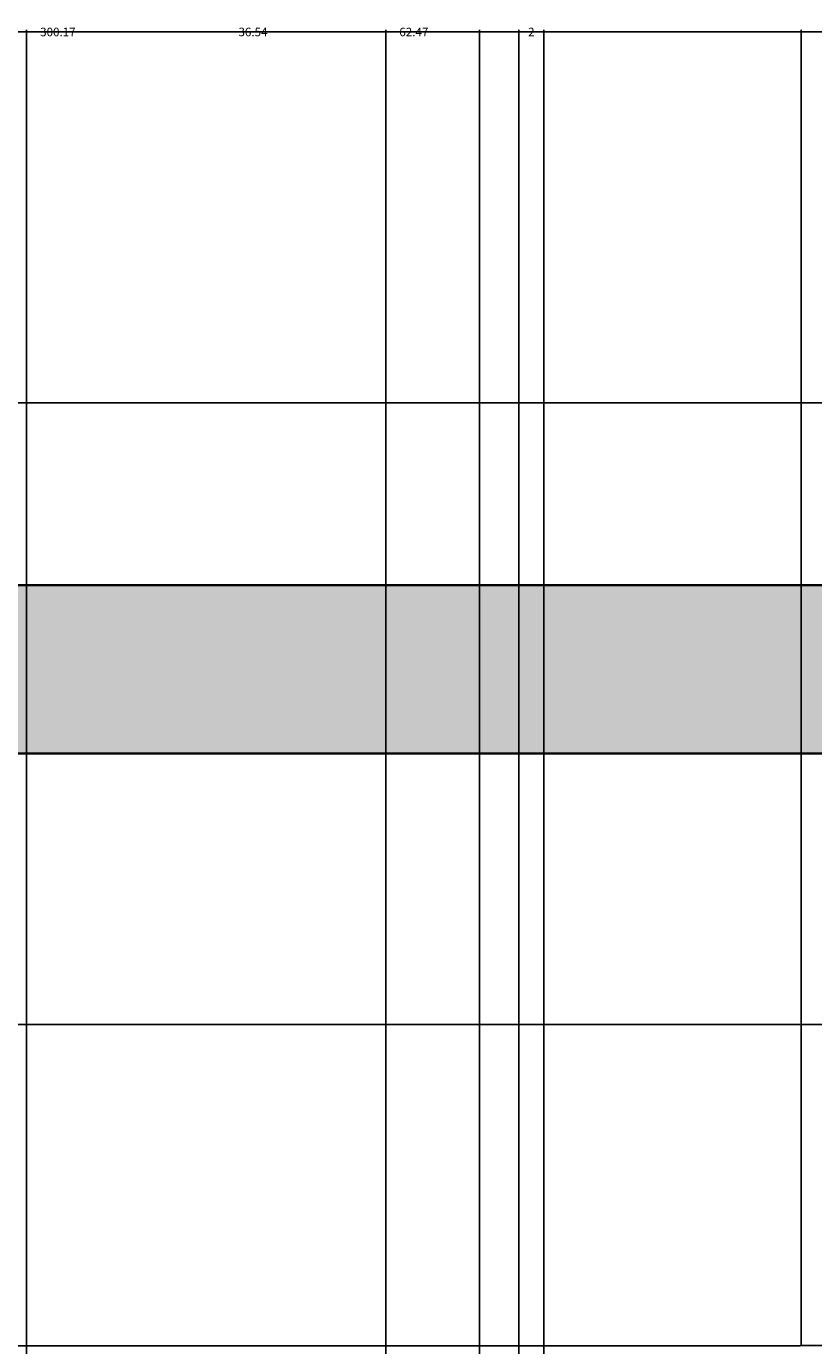
# Model space of a CAD drawing. Units: inches. Extents: x -145 to 510, y 5 to 386.
# Tile 21 of 25: x 182 to 245, y 280 to 386. Entities that reach past the tile are written whole.
import ezdxf

# ---------------------------------------------------------------- set-up
doc = ezdxf.new("R2010")
doc.units = ezdxf.units.IN
doc.header["$MEASUREMENT"] = 0
for name, color, linetype, lineweight in [('A-ANNO-DIMS', 2, 'Continuous', 18), ('A-ELEV', 7, 'Continuous', 35), ('A-ELEV-PATT', 8, 'Continuous', 13), ('A-GLAZ', 4, 'Continuous', 25)]:
    doc.layers.add(name, color=color, linetype=linetype, lineweight=lineweight)
doc.styles.get("Standard").update_dxf_attribs({"font": 'arial.ttf'})
doc.dimstyles.get("Standard").update_dxf_attribs({"dimtxt": 0.6875, "dimasz": 0.18, "dimexe": 0.18, "dimexo": 0.0625, "dimgap": 0.09, "dimtad": 0, "dimtih": 1, "dimtoh": 1, "dimdec": 4, "dimzin": 0, "dimdsep": 46, "dimlunit": 4, "dimtxsty": 'Standard', "dimcen": 0.09, "dimadec": 0, "dimazin": 0, "dimtfac": 1, "dimtdec": 4, "dimtofl": 0, "dimtmove": 0, "dimatfit": 3, "dimfxl": 1, "dimtolj": 1, "dimtzin": 0, "dimarcsym": 0})

# ---------------------------------------------------------------- blocks, each defined once
blk = doc.blocks.new('*D14')
at = {"layer": 'A-ANNO-DIMS', "color": 0, "lineweight": -2, "transparency": 16777216}
for p, q in [((34.27, 341.23), (34.27, 385.97)), ((34.45, 385.79), (255.28, 385.79)), ((478.65, 385.79), (257.81, 385.79)), ((478.83, 355.95), (478.83, 385.97))]:
    blk.add_line(p, q, dxfattribs=at)
at = {"layer": 'A-ANNO-DIMS', "color": 0, "transparency": 16777216}
for points in [[(34.45, 385.82), (34.45, 385.76), (34.27, 385.79)], [(478.65, 385.82), (478.65, 385.76), (478.83, 385.79)]]:
    blk.add_solid(points, dxfattribs=at)
at = {"layer": 'Defpoints', "color": 0, "transparency": 16777216}
for p in [(478.83, 385.79), (478.83, 355.89), (34.27, 341.17)]:
    blk.add_point(p, dxfattribs=at)
at = {"layer": 'A-ANNO-DIMS', "color": 0, "transparency": 16777216, "insert": (256.55, 385.79), "char_height": 0.688, "attachment_point": 5}
blk.add_mtext('\\A1;444.6', dxfattribs=at)
blk = doc.blocks.new('*D16')
at = {"layer": 'A-ANNO-DIMS', "color": 0, "lineweight": -2, "transparency": 16777216}
for p, q in [((95.14, 305.8), (95.14, 385.97)), ((95.32, 385.79), (137.23, 385.79)), ((181.64, 385.79), (139.73, 385.79)), ((181.82, 305.8), (181.82, 385.97))]:
    blk.add_line(p, q, dxfattribs=at)
at = {"layer": 'A-ANNO-DIMS', "color": 0, "transparency": 16777216}
for points in [[(95.32, 385.82), (95.32, 385.76), (95.14, 385.79)], [(181.64, 385.82), (181.64, 385.76), (181.82, 385.79)]]:
    blk.add_solid(points, dxfattribs=at)
at = {"layer": 'Defpoints', "color": 0, "transparency": 16777216}
for p in [(181.82, 385.79), (95.14, 305.74), (181.82, 305.74)]:
    blk.add_point(p, dxfattribs=at)
at = {"layer": 'A-ANNO-DIMS', "color": 0, "transparency": 16777216, "insert": (138.48, 385.79), "char_height": 0.688, "attachment_point": 5}
blk.add_mtext('\\A1;86.68', dxfattribs=at)
blk = doc.blocks.new('*D17')
at = {"layer": 'A-ANNO-DIMS', "color": 0, "lineweight": -2, "transparency": 16777216}
for p, q in [((181.82, 305.8), (181.82, 385.97)), ((182, 385.79), (211.8, 385.79)), ((244.11, 385.79), (214.31, 385.79)), ((244.29, 305.8), (244.29, 385.97))]:
    blk.add_line(p, q, dxfattribs=at)
at = {"layer": 'A-ANNO-DIMS', "color": 0, "transparency": 16777216}
for points in [[(182, 385.82), (182, 385.76), (181.82, 385.79)], [(244.11, 385.82), (244.11, 385.76), (244.29, 385.79)]]:
    blk.add_solid(points, dxfattribs=at)
at = {"layer": 'Defpoints', "color": 0, "transparency": 16777216}
for p in [(244.29, 385.79), (181.82, 305.74), (244.29, 305.74)]:
    blk.add_point(p, dxfattribs=at)
at = {"layer": 'A-ANNO-DIMS', "color": 0, "transparency": 16777216, "insert": (213.06, 385.79), "char_height": 0.688, "attachment_point": 5}
blk.add_mtext('\\A1;62.47', dxfattribs=at)
blk = doc.blocks.new('*D18')
at = {"layer": 'A-ANNO-DIMS', "color": 0, "lineweight": -2, "transparency": 16777216}
for p, q in [((244.29, 305.8), (244.29, 385.97)), ((244.47, 385.79), (268.26, 385.79)), ((294.56, 385.79), (270.77, 385.79)), ((294.74, 305.8), (294.74, 385.97))]:
    blk.add_line(p, q, dxfattribs=at)
at = {"layer": 'A-ANNO-DIMS', "color": 0, "transparency": 16777216}
for points in [[(244.47, 385.82), (244.47, 385.76), (244.29, 385.79)], [(294.56, 385.82), (294.56, 385.76), (294.74, 385.79)]]:
    blk.add_solid(points, dxfattribs=at)
at = {"layer": 'Defpoints', "color": 0, "transparency": 16777216}
for p in [(294.74, 385.79), (244.29, 305.74), (294.74, 305.74)]:
    blk.add_point(p, dxfattribs=at)
at = {"layer": 'A-ANNO-DIMS', "color": 0, "transparency": 16777216, "insert": (269.51, 385.79), "char_height": 0.688, "attachment_point": 5}
blk.add_mtext('\\A1;50.45', dxfattribs=at)
blk = doc.blocks.new('*D19')
at = {"layer": 'A-ANNO-DIMS', "color": 0, "lineweight": -2, "transparency": 16777216}
for p, q in [((478.76, 355.89), (-144.05, 355.89)), ((-143.87, 355.71), (-143.87, 218.33)), ((-143.87, 80.07), (-143.87, 217.45)), ((-114.04, 79.89), (-144.05, 79.89))]:
    blk.add_line(p, q, dxfattribs=at)
at = {"layer": 'A-ANNO-DIMS', "color": 0, "transparency": 16777216}
for points in [[(-143.9, 355.71), (-143.84, 355.71), (-143.87, 355.89)], [(-143.9, 80.07), (-143.84, 80.07), (-143.87, 79.89)]]:
    blk.add_solid(points, dxfattribs=at)
at = {"layer": 'Defpoints', "color": 0, "transparency": 16777216}
for p in [(-143.87, 355.89), (478.83, 355.89), (-113.97, 79.89)]:
    blk.add_point(p, dxfattribs=at)
at = {"layer": 'A-ANNO-DIMS', "color": 0, "transparency": 16777216, "insert": (-143.87, 217.89), "char_height": 0.688, "attachment_point": 5}
blk.add_mtext('\\A1;276', dxfattribs=at)
blk = doc.blocks.new('*D28')
at = {"layer": 'A-ANNO-DIMS', "color": 0, "lineweight": -2, "transparency": 16777216}
for p, q in [((244.23, 305.74), (-144.05, 305.74)), ((-143.87, 305.56), (-143.87, 293.23)), ((-143.87, 280.02), (-143.87, 292.35)), ((244.23, 279.84), (-144.05, 279.84))]:
    blk.add_line(p, q, dxfattribs=at)
at = {"layer": 'A-ANNO-DIMS', "color": 0, "transparency": 16777216}
for points in [[(-143.9, 305.56), (-143.84, 305.56), (-143.87, 305.74)], [(-143.9, 280.02), (-143.84, 280.02), (-143.87, 279.84)]]:
    blk.add_solid(points, dxfattribs=at)
at = {"layer": 'Defpoints', "color": 0, "transparency": 16777216}
for p in [(-143.87, 305.74), (244.29, 305.74), (244.29, 279.84)]:
    blk.add_point(p, dxfattribs=at)
at = {"layer": 'A-ANNO-DIMS', "color": 0, "transparency": 16777216, "insert": (-143.87, 292.79), "char_height": 0.688, "attachment_point": 5}
blk.add_mtext('\\A1;25.897', dxfattribs=at)
blk = doc.blocks.new('*D43')
at = {"layer": 'A-ANNO-DIMS', "color": 0, "lineweight": -2, "transparency": 16777216}
for p, q in [((34.27, 341.23), (34.27, 385.97)), ((34.45, 385.79), (182.84, 385.79)), ((334.26, 385.79), (185.87, 385.79)), ((334.44, 327.67), (334.44, 385.97))]:
    blk.add_line(p, q, dxfattribs=at)
at = {"layer": 'A-ANNO-DIMS', "color": 0, "transparency": 16777216}
for points in [[(34.45, 385.82), (34.45, 385.76), (34.27, 385.79)], [(334.26, 385.82), (334.26, 385.76), (334.44, 385.79)]]:
    blk.add_solid(points, dxfattribs=at)
at = {"layer": 'Defpoints', "color": 0, "transparency": 16777216}
for p in [(334.44, 385.79), (34.27, 341.17), (334.44, 327.61)]:
    blk.add_point(p, dxfattribs=at)
at = {"layer": 'A-ANNO-DIMS', "color": 0, "transparency": 16777216, "insert": (184.36, 385.79), "char_height": 0.688, "attachment_point": 5}
blk.add_mtext('\\A1;300.17', dxfattribs=at)
blk = doc.blocks.new('*D45')
at = {"layer": 'A-ANNO-DIMS', "color": 0, "lineweight": -2, "transparency": 16777216}
for p, q in [((210.8, 188.37), (210.8, 385.97)), ((210.98, 385.79), (262.53, 385.79)), ((317.05, 385.79), (265.5, 385.79)), ((317.23, 178.08), (317.23, 385.97))]:
    blk.add_line(p, q, dxfattribs=at)
at = {"layer": 'A-ANNO-DIMS', "color": 0, "transparency": 16777216}
for points in [[(210.98, 385.82), (210.98, 385.76), (210.8, 385.79)], [(317.05, 385.82), (317.05, 385.76), (317.23, 385.79)]]:
    blk.add_solid(points, dxfattribs=at)
at = {"layer": 'Defpoints', "color": 0, "transparency": 16777216}
for p in [(317.23, 385.79), (210.8, 188.31), (317.23, 178.02)]:
    blk.add_point(p, dxfattribs=at)
at = {"layer": 'A-ANNO-DIMS', "color": 0, "transparency": 16777216, "insert": (264.01, 385.79), "char_height": 0.688, "attachment_point": 5}
blk.add_mtext('\\A1;106.43', dxfattribs=at)
blk = doc.blocks.new('*D46')
at = {"layer": 'A-ANNO-DIMS', "color": 0, "lineweight": -2, "transparency": 16777216}
for p, q in [((181.82, 199.95), (181.82, 385.97)), ((182, 385.79), (198.84, 385.79)), ((218.18, 385.79), (201.34, 385.79)), ((218.36, 199.95), (218.36, 385.97))]:
    blk.add_line(p, q, dxfattribs=at)
at = {"layer": 'A-ANNO-DIMS', "color": 0, "transparency": 16777216}
for points in [[(182, 385.82), (182, 385.76), (181.82, 385.79)], [(218.18, 385.82), (218.18, 385.76), (218.36, 385.79)]]:
    blk.add_solid(points, dxfattribs=at)
at = {"layer": 'Defpoints', "color": 0, "transparency": 16777216}
for p in [(218.36, 385.79), (181.82, 199.89), (218.36, 199.89)]:
    blk.add_point(p, dxfattribs=at)
at = {"layer": 'A-ANNO-DIMS', "color": 0, "transparency": 16777216, "insert": (200.09, 385.79), "char_height": 0.688, "attachment_point": 5}
blk.add_mtext('\\A1;36.54', dxfattribs=at)
blk = doc.blocks.new('*D50')
at = {"layer": 'A-ANNO-DIMS', "color": 0, "lineweight": -2, "transparency": 16777216}
for p, q in [((221.53, 156.67), (221.53, 385.97)), ((221.71, 385.79), (246.26, 385.79)), ((273.31, 385.79), (248.76, 385.79)), ((273.49, 156.67), (273.49, 385.97))]:
    blk.add_line(p, q, dxfattribs=at)
at = {"layer": 'A-ANNO-DIMS', "color": 0, "transparency": 16777216}
for points in [[(221.71, 385.82), (221.71, 385.76), (221.53, 385.79)], [(273.31, 385.82), (273.31, 385.76), (273.49, 385.79)]]:
    blk.add_solid(points, dxfattribs=at)
at = {"layer": 'Defpoints', "color": 0, "transparency": 16777216}
for p in [(273.49, 385.79), (221.53, 156.61), (273.49, 156.61)]:
    blk.add_point(p, dxfattribs=at)
at = {"layer": 'A-ANNO-DIMS', "color": 0, "transparency": 16777216, "insert": (247.51, 385.79), "char_height": 0.688, "attachment_point": 5}
blk.add_mtext('\\A1;51.96', dxfattribs=at)
blk = doc.blocks.new('*D53')
at = {"layer": 'A-ANNO-DIMS', "color": 0, "lineweight": -2, "transparency": 16777216}
for p, q in [((221.53, 85.33), (221.53, 385.97)), ((221.71, 385.79), (222.21, 385.79)), ((223.35, 385.79), (222.85, 385.79)), ((223.53, 87.33), (223.53, 385.97))]:
    blk.add_line(p, q, dxfattribs=at)
at = {"layer": 'A-ANNO-DIMS', "color": 0, "transparency": 16777216}
for points in [[(221.71, 385.82), (221.71, 385.76), (221.53, 385.79)], [(223.35, 385.82), (223.35, 385.76), (223.53, 385.79)]]:
    blk.add_solid(points, dxfattribs=at)
at = {"layer": 'Defpoints', "color": 0, "transparency": 16777216}
for p in [(223.53, 385.79), (223.53, 87.26), (221.53, 85.26)]:
    blk.add_point(p, dxfattribs=at)
at = {"layer": 'A-ANNO-DIMS', "color": 0, "transparency": 16777216, "insert": (222.53, 385.79), "char_height": 0.688, "attachment_point": 5}
blk.add_mtext('\\A1;2', dxfattribs=at)

msp = doc.modelspace()

# ---------------------------------------------------------------- hatches: boundary and pattern name
at = {"layer": 'A-ELEV-PATT'}
h = msp.add_hatch(color=256, dxfattribs=at)
h.dxf.hatch_style = 1
h.paths.add_polyline_path([(334.4402, 341.168), (69.7763, 341.168), (69.7763, 327.6093), (334.4402, 327.6093)])
h.paths.add_polyline_path([(69.7763, 341.168), (34.2706, 341.168), (34.2706, 327.6093), (69.7763, 327.6093)])
h.paths.add_polyline_path([(317.2273, 188.3087), (210.7973, 188.3087), (210.7973, 178.0195), (317.2273, 178.0195)])
h.paths.add_polyline_path([(474.4893, 235.8905), (317.2273, 235.8905), (317.2273, 223.8905), (474.4893, 223.8905)])
h.paths.add_polyline_path([(317.2273, 235.8905), (309.4739, 235.8905), (309.4739, 223.8905), (317.2273, 223.8905)])
h.paths.add_polyline_path([(478.8263, 235.8905), (474.4893, 235.8905), (474.4893, 223.8905), (478.8263, 223.8905)])

# ---------------------------------------------------------------- linework, layer by layer
at = {"layer": 'A-ELEV'}
for p, q in [((69.7763, 341.168), (334.4402, 341.168)), ((34.2706, 327.6093), (334.4402, 327.6093))]:
    msp.add_line(p, q, dxfattribs=at)
at = {"layer": 'A-GLAZ'}
msp.add_lwpolyline([(244.2916, 305.7416), (294.738, 305.7416), (294.738, 279.8443), (244.2916, 279.8443)], close=True, dxfattribs=at)

# ---------------------------------------------------------------- dimensions: what is measured, and where the dimension line sits
at = {"layer": 'A-ANNO-DIMS'}
for base, p1, p2, override, picture, middle in [((478.8263, 385.7905), (34.2706, 341.168), (478.8263, 355.8905), {"dimdec": 1, "dimlfac": 1, "dimrnd": 0, "dimzin": 0, "dimdsep": 46, "dimlunit": 2}, '*D14', (256.5484, 385.7905)), ((334.4402, 385.7905), (34.2706, 341.168), (334.4402, 327.6093), {"dimdec": 2, "dimlfac": 1, "dimrnd": 0, "dimzin": 0, "dimdsep": 46, "dimlunit": 2}, '*D43', (184.3554, 385.7905)), ((181.8195, 385.7905), (95.1414, 305.7416), (181.8195, 305.7416), {"dimdec": 2, "dimlfac": 1, "dimrnd": 0, "dimzin": 0, "dimdsep": 46, "dimlunit": 2}, '*D16', (138.4805, 385.7905)), ((244.2916, 385.7905), (181.8195, 305.7416), (244.2916, 305.7416), {"dimdec": 2, "dimlfac": 1, "dimrnd": 0, "dimzin": 0, "dimdsep": 46, "dimlunit": 2}, '*D17', (213.0556, 385.7905)), ((218.3571, 385.7905), (181.8195, 199.8905), (218.3571, 199.8905), {"dimdec": 2, "dimlfac": 1, "dimrnd": 0, "dimzin": 0, "dimdsep": 46, "dimlunit": 2}, '*D46', (200.0883, 385.7905)), ((317.2273, 385.7905), (210.7973, 188.3087), (317.2273, 178.0195), {"dimdec": 2, "dimlfac": 1, "dimrnd": 0, "dimzin": 0, "dimdsep": 46, "dimlunit": 2}, '*D45', (264.0123, 385.7905)), ((273.4905, 385.7905), (221.5292, 156.6093), (273.4905, 156.6093), {"dimdec": 2, "dimlfac": 1, "dimrnd": 0, "dimzin": 0, "dimdsep": 46, "dimlunit": 2}, '*D50', (247.5098, 385.7905)), ((223.5292, 385.7905), (221.5292, 85.2638), (223.5292, 87.2638), {"dimdec": 0, "dimlfac": 1, "dimrnd": 0, "dimzin": 0, "dimdsep": 46, "dimlunit": 2}, '*D53', (222.5292, 385.7905)), ((294.738, 385.7905), (244.2916, 305.7416), (294.738, 305.7416), {"dimdec": 2, "dimlfac": 1, "dimrnd": 0, "dimzin": 0, "dimdsep": 46, "dimlunit": 2}, '*D18', (269.5148, 385.7905))]:
    dim = msp.add_linear_dim(base=base, p1=p1, p2=p2, dimstyle='Standard', override=override, dxfattribs=at)
    dim.commit()
    dim.dimension.update_dxf_attribs({"geometry": picture, "text_midpoint": middle})
for base, p1, p2, override, picture, middle in [((-143.8737, 355.8905), (-113.9737, 79.8905), (478.8263, 355.8905), {"dimdec": 0, "dimlfac": 1, "dimrnd": 0, "dimzin": 0, "dimdsep": 46, "dimlunit": 2}, '*D19', (-143.8737, 217.8905)), ((-143.8737, 305.7416), (244.2916, 279.8443), (244.2916, 305.7416), {"dimdec": 3, "dimlfac": 1, "dimrnd": 0, "dimzin": 0, "dimdsep": 46, "dimlunit": 2}, '*D28', (-143.8737, 292.793))]:
    dim = msp.add_linear_dim(base=base, p1=p1, p2=p2, angle=90, dimstyle='Standard', override=override, dxfattribs=at)
    dim.commit()
    dim.dimension.update_dxf_attribs({"geometry": picture, "text_midpoint": middle})

doc.saveas('drawing.dxf')
